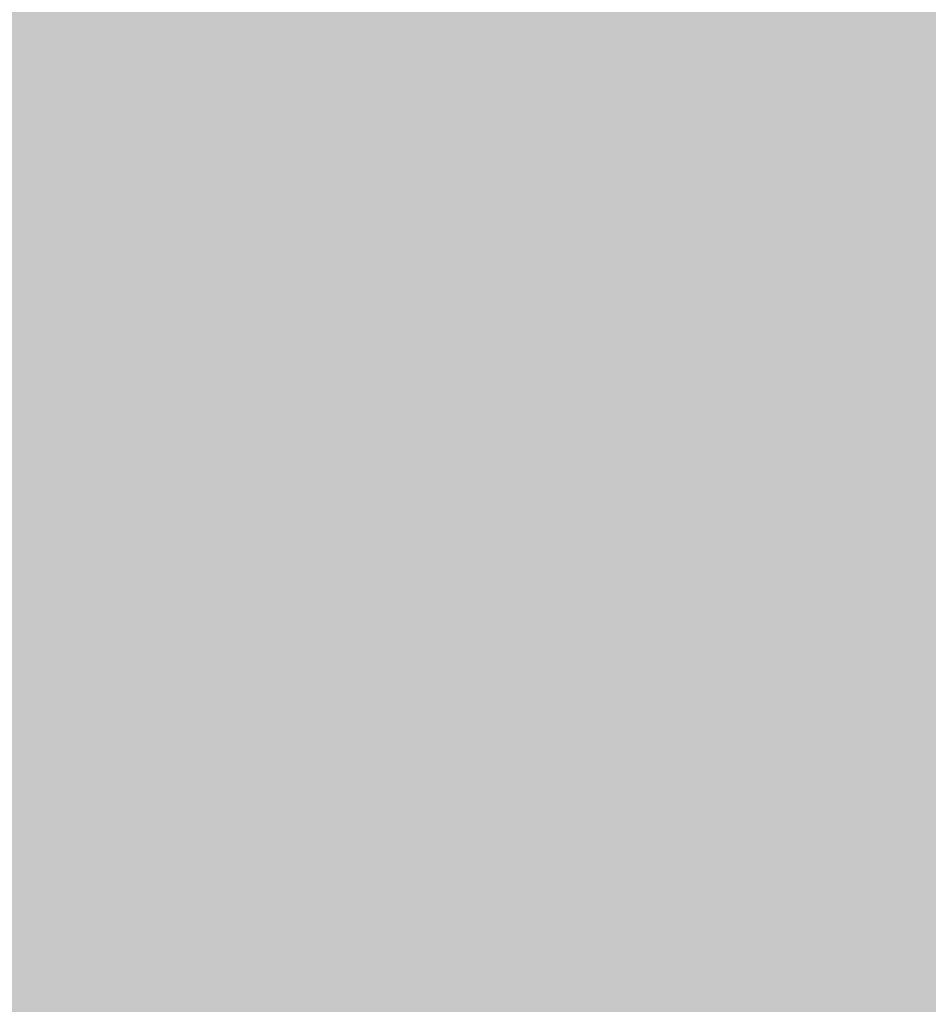
# Model space of a CAD drawing. Units: inches. Extents: x 1704 to 6393, y -157 to 1172.
# Tile 17 of 122: x 1934 to 1975, y 157 to 201. Entities that reach past the tile are written whole.
import ezdxf

# ---------------------------------------------------------------- set-up
doc = ezdxf.new("R2010")
doc.units = ezdxf.units.IN
doc.header["$MEASUREMENT"] = 0
doc.layers.add('A-ANNO-DIMS', color=7, linetype='Continuous', lineweight=13)
doc.layers.add('L-PLNT-PATT', color=253, linetype='Continuous', lineweight=13, true_color=0x9abc8f)
doc.styles.get("Standard").update_dxf_attribs({"font": 'arial.ttf'})
doc.dimstyles.get("Standard").update_dxf_attribs({"dimtxt": 6, "dimasz": 2, "dimexe": 0.18, "dimexo": 0.0625, "dimgap": 0.09, "dimtad": 0, "dimtih": 1, "dimtoh": 1, "dimdec": 1, "dimzin": 0, "dimdsep": 46, "dimlunit": 3, "dimtxsty": 'Standard', "dimblk": 'ARCHTICK', "dimcen": 0.09, "dimadec": 0, "dimazin": 0, "dimtfac": 1, "dimtdec": 1, "dimtofl": 0, "dimtmove": 0, "dimatfit": 3, "dimfxl": 1, "dimtolj": 1, "dimtzin": 0, "dimarcsym": 0})

# ---------------------------------------------------------------- blocks, each defined once
blk = doc.blocks.new('_ArchTick')
at = {"color": 0, "linetype": 'ByBlock', "const_width": 0.15}
blk.add_lwpolyline([(-0.5, -0.5), (0.5, 0.5)], dxfattribs=at)
blk = doc.blocks.new('*D93')
at = {"layer": 'A-ANNO-DIMS', "color": 0, "lineweight": -2, "transparency": 16777216}
for p, q in [((2605.286, 895.213), (1829.698, 895.213)), ((1829.878, 895.213), (1829.878, 495.866)), ((1829.878, 90.213), (1829.878, 489.56)), ((2605.286, 90.213), (1829.698, 90.213))]:
    blk.add_line(p, q, dxfattribs=at)
at = {"layer": 'Defpoints', "color": 0, "lineweight": -3, "transparency": 16777216}
for p in [(2605.349, 895.213), (1829.878, 90.213), (2605.349, 90.213)]:
    blk.add_point(p, dxfattribs=at)
at = {"layer": 'A-ANNO-DIMS', "color": 0, "lineweight": -2, "transparency": 16777216, "xscale": 2, "yscale": 2, "zscale": 2}
for p, rotation in [((1829.878, 895.213), 90), ((1829.878, 90.213), 270)]:
    blk.add_blockref('_ArchTick', p, dxfattribs=dict(at, rotation=rotation))
at = {"layer": 'A-ANNO-DIMS', "color": 0, "transparency": 16777216, "insert": (1829.878, 492.713), "char_height": 6, "attachment_point": 5}
blk.add_mtext('\\A1;805', dxfattribs=at)

msp = doc.modelspace()

# ---------------------------------------------------------------- hatches: boundary and pattern name
at = {"layer": 'L-PLNT-PATT', "transparency": 33554643}
h = msp.add_hatch(color=256, dxfattribs=at)
h.dxf.hatch_style = 1
h.paths.add_polyline_path([(1975.349, 202.213), (1898.349, 202.213), (1898.349, -3.787), (1975.349, -3.787)])

# ---------------------------------------------------------------- dimensions: what is measured, and where the dimension line sits
at = {"layer": 'A-ANNO-DIMS'}
dim = msp.add_linear_dim(base=(1829.878, 90.213), p1=(2605.349, 895.213), p2=(2605.349, 90.213), angle=90, dimstyle='Standard', override={"dimdec": 0, "dimlfac": 1, "dimrnd": 0, "dimzin": 0, "dimdsep": 46, "dimlunit": 2}, dxfattribs=at)
dim.commit()
dim.dimension.update_dxf_attribs({"geometry": '*D93', "text_midpoint": (1829.878, 492.713)})

doc.saveas('drawing.dxf')
